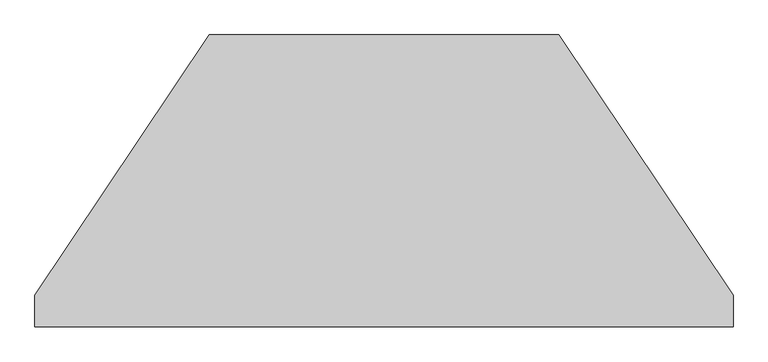
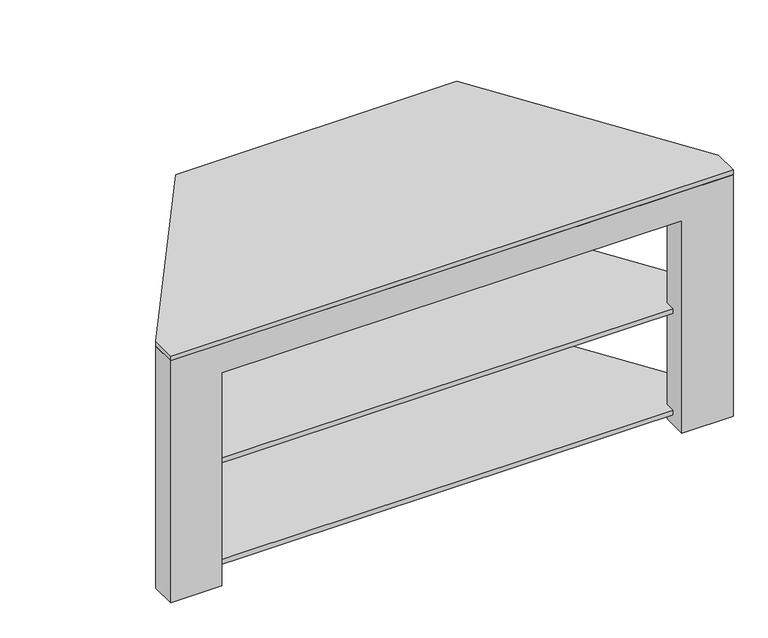
"""IFC4 building model written with IfcOpenShell, lengths in millimetres: furniture geometry."""

from ifc_helpers import new_model, si_unit, point, frame, frame_2d, origin, place, context, project, spatial, polyline, circle_curve, trimmed, segment, composite_curve, outline, extrude, faceted_brep, source, transform, mapped, element, save


def furniture_dc210597(model_context):
    return source(origin(), model_context, "Body", "SolidModel", [
        extrude(outline(polyline([(0.0, 300.1880021), (500.0, 300.1880021), (500.0, -49.8119979), (0.0, -49.8119979), (0.0, 300.1880021)]), holes=[composite_curve([segment(polyline([(245.0, 145.1700818), (245.0, 105.2059224)]), True, "CONTINUOUS"), segment(trimmed(circle_curve(frame_2d((257.5, 105.2059224)), 12.5), [point((245.0, 105.2059224))], [point((270.0, 105.2059224))], True, "CARTESIAN"), True, "CONTINUOUS"), segment(polyline([(270.0, 105.2059224), (270.0, 145.1700818)]), True, "CONTINUOUS"), segment(trimmed(circle_curve(frame_2d((257.5, 145.1700818)), 12.5), [point((270.0, 145.1700818))], [point((245.0, 145.1700818))], True, "CARTESIAN"), True, "CONTINUOUS")], self_intersect=False), composite_curve([segment(polyline([(35.0, 145.1880021), (35.0, 105.2059224)]), True, "CONTINUOUS"), segment(trimmed(circle_curve(frame_2d((47.5, 105.2059224)), 12.5), [point((35.0, 105.2059224))], [point((60.0, 105.2059224))], True, "CARTESIAN"), True, "CONTINUOUS"), segment(polyline([(60.0, 105.2059224), (60.0, 145.1880021)]), True, "CONTINUOUS"), segment(trimmed(circle_curve(frame_2d((47.5, 145.1880021)), 12.5), [point((60.0, 145.1880021))], [point((35.0, 145.1880021))], True, "CARTESIAN"), True, "CONTINUOUS")], self_intersect=False)]), frame((0.0, -30.0, 0.0), z_axis=(0.0, 1.0, 0.0), x_axis=(0.0, 0.0, 1.0)), (0.0, 0.0, 1.0), 10.0),
        faceted_brep([(-424.8119979, -460.0, 0.0), (-324.8119979, -460.0, 0.0), (-324.8119979, -460.0, 440.0), (575.1880021, -460.0, 440.0), (575.1880021, -460.0, 0.0), (675.1880021, -460.0, 0.0), (675.1880021, -460.0, 500.0), (-424.8119979, -460.0, 500.0), (-424.8119979, -410.0, 0.0), (-424.8119979, -410.0, 500.0), (675.1880021, -410.0, 500.0), (675.1880021, -410.0, 0.0), (575.1880021, -410.0, 0.0), (575.1880021, -410.0, 20.0), (625.1880021, -410.0, 20.0), (625.1880021, -410.0, 30.0), (575.1880021, -410.0, 30.0), (575.1880021, -410.0, 230.0), (625.1880021, -410.0, 230.0), (625.1880021, -410.0, 240.0), (575.1880021, -410.0, 240.0), (575.1880021, -410.0, 440.0), (-324.8119979, -410.0, 440.0), (-324.8119979, -410.0, 240.0), (-374.8119979, -410.0, 240.0), (-374.8119979, -410.0, 230.0), (-324.8119979, -410.0, 230.0), (-324.8119979, -410.0, 30.0), (-374.8119979, -410.0, 30.0), (-374.8119979, -410.0, 20.0), (-324.8119979, -410.0, 20.0), (-324.8119979, -410.0, 0.0), (-324.8119979, -430.0, 20.0), (-324.8119979, -430.0, 30.0), (-324.8119979, -430.0, 230.0), (-324.8119979, -430.0, 240.0), (575.1880021, -430.0, 240.0), (575.1880021, -430.0, 230.0), (575.1880021, -430.0, 30.0), (575.1880021, -430.0, 20.0), (625.1880021, -430.0, 240.0), (-374.8119979, -430.0, 240.0), (-374.8119979, -430.0, 230.0), (625.1880021, -430.0, 230.0), (625.1880021, -430.0, 30.0), (-374.8119979, -430.0, 30.0), (-374.8119979, -430.0, 20.0), (625.1880021, -430.0, 20.0)], [[[0, 1, 2, 3, 4, 5, 6, 7]], [[8, 9, 10, 11, 12, 13, 14, 15, 16, 17, 18, 19, 20, 21, 22, 23, 24, 25, 26, 27, 28, 29, 30, 31]], [[1, 0, 8, 31]], [[2, 1, 31, 30, 32, 33, 27, 26, 34, 35, 23, 22]], [[3, 2, 22, 21]], [[4, 3, 21, 20, 36, 37, 17, 16, 38, 39, 13, 12]], [[5, 4, 12, 11]], [[6, 5, 11, 10]], [[7, 6, 10, 9]], [[0, 7, 9, 8]], [[19, 40, 36, 20]], [[35, 41, 24, 23]], [[25, 42, 34, 26]], [[37, 43, 18, 17]], [[41, 42, 25, 24]], [[42, 41, 35, 34]], [[40, 43, 37, 36]], [[43, 40, 19, 18]], [[15, 44, 38, 16]], [[33, 45, 28, 27]], [[29, 46, 32, 30]], [[39, 47, 14, 13]], [[45, 46, 29, 28]], [[46, 45, 33, 32]], [[44, 47, 39, 38]], [[47, 44, 15, 14]]]),
        extrude(outline(polyline([(-50.0, 500.0), (0.0, 500.0), (0.0, 0.0), (-50.0, 0.0), (-50.0, 20.0), (-30.0, 20.0), (-30.0, 30.0), (-50.0, 30.0), (-50.0, 230.0), (-30.0, 230.0), (-30.0, 240.0), (-50.0, 240.0), (-50.0, 500.0)])), frame((-149.8119979, 0.0, 0.0), z_axis=(1.0, 0.0, 0.0), x_axis=(0.0, 1.0, 0.0)), (0.0, 0.0, 1.0), 100.0),
        extrude(outline(polyline([(-50.0, 500.0), (0.0, 500.0), (0.0, 0.0), (-50.0, 0.0), (-50.0, 20.0), (-30.0, 20.0), (-30.0, 30.0), (-50.0, 30.0), (-50.0, 230.0), (-30.0, 230.0), (-30.0, 240.0), (-50.0, 240.0), (-50.0, 500.0)])), frame((300.1880021, 0.0, 0.0), z_axis=(1.0, 0.0, 0.0), x_axis=(0.0, 1.0, 0.0)), (0.0, 0.0, 1.0), 100.0),
        extrude(outline(polyline([(400.1880021, 0.0), (675.1880021, -410.0), (675.1880021, -460.0), (-424.8119979, -460.0), (-424.8119979, -410.0), (-149.8119979, 0.0), (400.1880021, 0.0)])), frame((0.0, 0.0, 500.0), z_axis=(0.0, 0.0, 1.0), x_axis=(1.0, 0.0, 0.0)), (0.0, 0.0, 1.0), 10.0),
        extrude(outline(polyline([(420.3099533, -30.0), (625.1880021, -335.4545455), (625.1880021, -430.0), (-374.8119979, -430.0), (-374.8119979, -335.4545455), (-169.9339492, -30.0), (420.3099533, -30.0)])), frame((0.0, 0.0, 230.0), z_axis=(0.0, 0.0, 1.0), x_axis=(1.0, 0.0, 0.0)), (0.0, 0.0, 1.0), 10.0),
        extrude(outline(polyline([(420.3099533, -30.0), (625.1880021, -335.4545455), (625.1880021, -430.0), (-374.8119979, -430.0), (-374.8119979, -335.4545455), (-169.9339492, -30.0), (420.3099533, -30.0)])), frame((0.0, 0.0, 20.0), z_axis=(0.0, 0.0, 1.0), x_axis=(1.0, 0.0, 0.0)), (0.0, 0.0, 1.0), 10.0),
    ])


if __name__ == "__main__":
    model = new_model("IFC4")
    model_context = context("Model", 3, world=origin())
    ifc_project = project(units=[si_unit("LENGTHUNIT", "METRE", prefix="MILLI")], contexts=[model_context])
    site = spatial("IfcSite", under=ifc_project)
    building = spatial("IfcBuilding", under=site)
    placement = place(None, origin())
    furniture_shape = furniture_dc210597(model_context)
    element("IfcFurniture", 1, at=placement, inside=building, context=model_context, shape_type="MappedRepresentation", body=[
        mapped(furniture_shape, transform((0.0, 0.0, 0.0), x_axis=(1.0, 0.0, 0.0), y_axis=(0.0, 1.0, 0.0), z_axis=(0.0, 0.0, 1.0))),
    ])
    save(model, "model.ifc")

# Revit data of these elements
# Type
#   Depth = 1.509186 ft
#   Width = 3.608924 ft
#   Height = 1.64042 ft
#   Finish = Melamine - Gray
#   Default Elevation = 0
# Element 1 (IfcFurniture)
#   Materials on its faces: "Melamine - Gray", "Glass - Shelves"
# Materials
#   "Melamine - Gray": class "Wood", colour RGB 49 49 49, transparency 0
#   "Glass - Shelves": class "Glass", colour RGB 167 167 167, transparency 0.9
